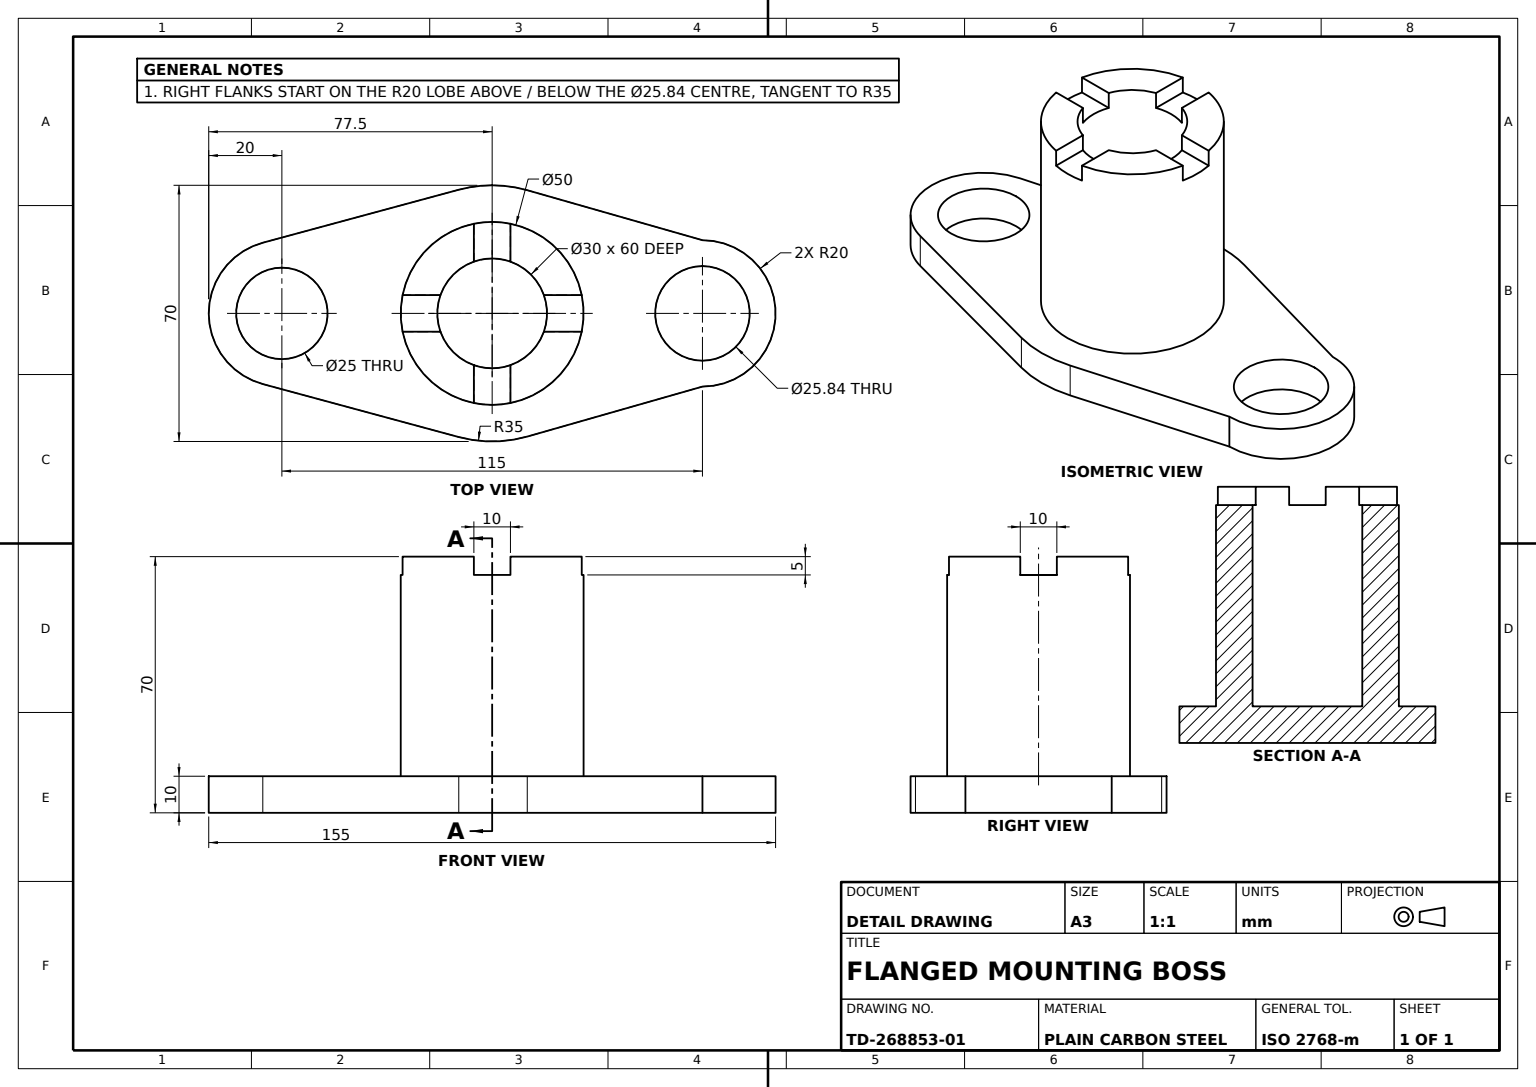
from build123d import *

# Parameters (mm, degrees)
FLANGE_PROFILE_R       = 12.5
FLANGE_PROFILE_R_2     = 12.920835642
FLANGE_PLATE_DEPTH     = 5
HUB_PROFILE_R          = 25
HUB_PROFILE_R_2        = 15
HUB_50_BORE_30_DEPTH   = 60
CROSS_SLOT_PROFILE_W   = 10
CROSS_SLOT_PROFILE_H   = 10.92
CROSS_SLOT_PROFILE_W_2 = 10.92
CROSS_SLOT_PROFILE_H_2 = 10
CROSS_SLOTS_4X10_DEPTH = 5


with BuildPart() as part:
    # Flange Profile → Flange Plate (new, symmetric)
    with BuildSketch(Plane(origin=(0, 0, 0), x_dir=(1, 0, 0), z_dir=(0, 1, 0))):
        with BuildLine():
            Line((-62.717391304, 19.30748114), (-9.130434783, 33.788091995))
            ThreePointArc((-9.130434783, 33.788091995), (0.242124563, 34.9991625), (9.597031237, 33.658535195))
            Line((9.597031237, 33.658535195), (57.5, 20))
            ThreePointArc((57.5, 20), (77.5, 0), (57.5, -20))
            Line((57.5, -20), (9.597031237, -33.658535195))
            ThreePointArc((9.597031237, -33.658535195), (0.242124563, -34.9991625), (-9.130434783, -33.788091995))
            Line((-9.130434783, -33.788091995), (-62.717391304, -19.30748114))
            ThreePointArc((-62.717391304, -19.30748114), (-77.5, 0), (-62.717391304, 19.30748114))
        make_face()
        with Locations(Location((-57.5, 0, 0), (0, 0, 270))):
            Circle(FLANGE_PROFILE_R, mode=Mode.SUBTRACT)
        with Locations(Location((57.5, 0, 0), (0, 0, 270))):
            Circle(FLANGE_PROFILE_R_2, mode=Mode.SUBTRACT)
    extrude(amount=FLANGE_PLATE_DEPTH, both=True)

    # Hub Profile → Hub Ø50 Bore Ø30 (add)
    with BuildSketch(Plane(origin=(0, 5, 0), x_dir=(1, 0, 0), z_dir=(0, 1, 0))):
        with Locations(Location((0, 0, 0), (0, 0, 270))):
            Circle(HUB_PROFILE_R)
        with Locations(Location((0, 0, 0), (0, 0, 270))):
            Circle(HUB_PROFILE_R_2, mode=Mode.SUBTRACT)
    extrude(amount=HUB_50_BORE_30_DEPTH)

    # Cross Slot Profile → Cross Slots 4x10 (cut)
    with BuildSketch(Plane(origin=(0, 65, 0), x_dir=(1, 0, 0), z_dir=(0, 1, 0))):
        with Locations((0, 19.602135624)):
            Rectangle(CROSS_SLOT_PROFILE_W, CROSS_SLOT_PROFILE_H)
        with Locations((19.602135624, 0)):
            Rectangle(CROSS_SLOT_PROFILE_W_2, CROSS_SLOT_PROFILE_H_2)
        with Locations((0, -19.602135624)):
            Rectangle(CROSS_SLOT_PROFILE_W, CROSS_SLOT_PROFILE_H)
        with Locations((-19.602135624, 0)):
            Rectangle(CROSS_SLOT_PROFILE_W_2, CROSS_SLOT_PROFILE_H_2)
    extrude(amount=-CROSS_SLOTS_4X10_DEPTH, mode=Mode.SUBTRACT)


solid = part.part
